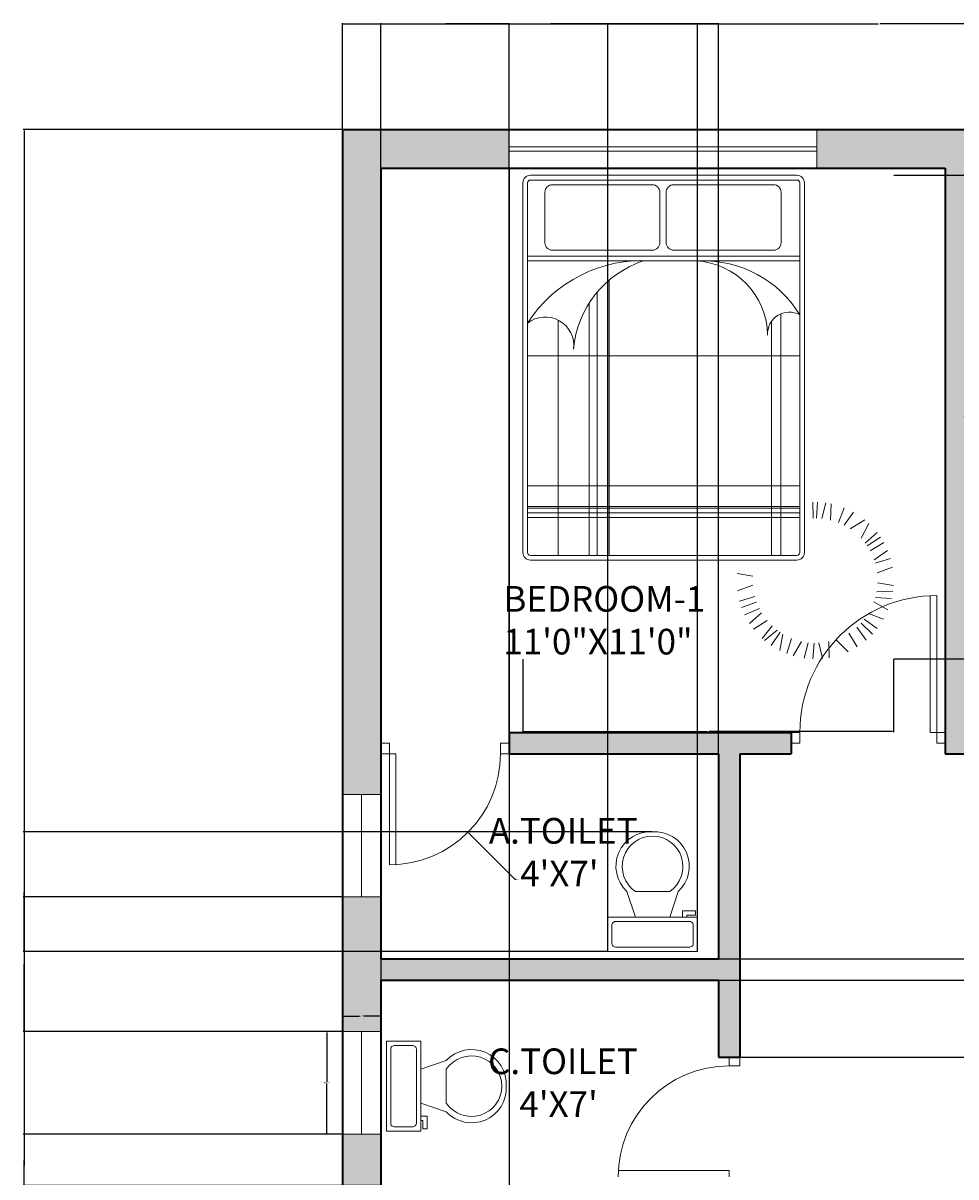
# Model space of a CAD drawing. Units: inches. Extents: x 126 to 477, y -70 to 465.
# Tile 3 of 5: x 126 to 344, y 195 to 465. Entities that reach past the tile are written whole.
import ezdxf

# ---------------------------------------------------------------- set-up
doc = ezdxf.new("R2010")
doc.units = ezdxf.units.IN
for name, color, linetype, lineweight in [('A-ANNO-DIMS', 2, 'Continuous', 18), ('A-AREA-IDEN', 7, 'Continuous', 20), ('A-DOOR', 4, 'Continuous', 20), ('A-FLOR-FIXT', 8, 'Continuous', 18), ('A-FURN', 8, 'Continuous', 18), ('A-GLAZ', 4, 'Continuous', 18), ('A-WALL', 7, 'Continuous', 35), ('A-WALL-PATT', 252, 'Continuous', 13)]:
    doc.layers.add(name, color=color, linetype=linetype, lineweight=lineweight)
doc.styles.get("Standard").update_dxf_attribs({"font": 'arial.ttf'})
doc.dimstyles.get("Standard").update_dxf_attribs({"dimtxt": 0.18, "dimasz": 0.18, "dimexe": 0.18, "dimexo": 0.0625, "dimgap": 0.09, "dimtad": 0, "dimtih": 1, "dimtoh": 1, "dimdec": 4, "dimzin": 0, "dimdsep": 46, "dimtxsty": 'Standard', "dimcen": 0.09, "dimadec": 0, "dimazin": 0, "dimtfac": 1, "dimtdec": 4, "dimtofl": 0, "dimtmove": 0, "dimatfit": 3, "dimfxl": 1, "dimtolj": 1, "dimtzin": 0, "dimarcsym": 0})

# ---------------------------------------------------------------- blocks, each defined once
blk = doc.blocks.new('*U6')
for p, q in [((9.5, -6), (9.5, -2)), ((-8, -8.5), (-8, -8)), ((-7, -8), (-7, -9.5)), ((-4, -8), (-6, -14)), ((4, -8), (6, -14)), ((-10, -8.5), (-8, -8.5)), ((-10, -9.5), (-10, -8.5)), ((-7, -9.5), (-10, -9.5)), ((4, -14), (-4, -14))]:
    blk.add_line(p, q)
blk.add_lwpolyline([(10.5, -8), (10.5, 0), (-10.5, 0), (-10.5, -8)], close=True)
for points in [[(-9.5, -2), (-9.5, -6)], [(8.5, -1), (-8.5, -1)], [(-8.5, -7), (8.5, -7)]]:
    blk.add_lwpolyline(points)
for centre, radius, start, end in [((-8.625, -1.875), 0.8839, 81.8699, 188.1301), ((8.625, -1.875), 0.8839, 351.8699, 98.1301), ((-8.625, -6.125), 0.8839, 171.869898, 278.1301), ((8.625, -6.125), 0.8839, 261.8699, 8.1301), ((-0.4772, -19.9188), 8.0953, 133.01722, 273.38), ((0.0374, -19.8731), 7.127, 124.50543, 269.7), ((-0.0373, -19.8731), 7.127, 270.3, 55.4946), ((0.4773, -19.9188), 8.0953, 266.62, 46.9828)]:
    blk.add_arc(centre, radius, start, end)
blk = doc.blocks.new('A$C20A07B91')
for p, q in [((0, 0.5668), (0, 2.5368)), ((0.025, 0.5668), (0.025, 2.5368)), ((0.04, 2.5768), (1.46, 2.5768)), ((0.04, 2.5518), (1.46, 2.5518)), ((0.1577, 2.5267), (0.6896, 2.5267)), ((0.8032, 2.5267), (1.3351, 2.5267)), ((1.475, 2.5368), (1.475, 0.5668)), ((1.5, 2.5368), (1.5, 0.5668)), ((0.1177, 2.2177), (0.1177, 2.4867)), ((0.7296, 2.4867), (0.7296, 2.2177)), ((0.7632, 2.2177), (0.7632, 2.4867)), ((1.3751, 2.4867), (1.3751, 2.2177)), ((0.6896, 2.1777), (0.1577, 2.1777)), ((1.3351, 2.1777), (0.8032, 2.1777)), ((1.475, 2.1455), (0.025, 2.1455)), ((1.475, 2.1208), (0.025, 2.1208)), ((0.4594, 2.0186), (0.4594, 0.5518)), ((0.3952, 1.9538), (0.3952, 0.5518)), ((0.3537, 1.8973), (0.3537, 0.5518)), ((0.1881, 1.8055), (0.1881, 0.5518)), ((1.325, 1.7998), (1.325, 0.5518)), ((1.3735, 1.8387), (1.3735, 0.5518)), ((1.475, 1.6146), (0.025, 1.6146)), ((1.475, 0.9216), (0.025, 0.9216)), ((1.475, 0.8127), (0.025, 0.8127)), ((1.475, 0.8028), (0.025, 0.8028)), ((1.5448, 0.8348), (1.5455, 0.7499)), ((1.5699, 0.8347), (1.5633, 0.7501)), ((1.6143, 0.831), (1.5932, 0.7481)), ((1.6427, 0.8261), (1.6378, 0.7402)), ((1.7121, 0.8051), (1.6806, 0.7263)), ((1.475, 0.778), (0.025, 0.778)), ((1.475, 0.7533), (0.025, 0.7533)), ((1.7614, 0.7816), (1.7107, 0.7125)), ((1.8218, 0.7404), (1.7431, 0.6933)), ((1.8424, 0.7223), (1.8011, 0.6437)), ((1.8863, 0.6743), (1.8232, 0.6171)), ((1.9045, 0.6491), (1.833, 0.6034)), ((1.9224, 0.6197), (1.8494, 0.5764)), ((1.9429, 0.5771), (1.8708, 0.5282)), ((1.46, 0.5518), (0.04, 0.5518)), ((1.46, 0.5268), (0.04, 0.5268)), ((1.9576, 0.5356), (1.8768, 0.5097)), ((1.1413, 0.4558), (1.2253, 0.4415)), ((1.9686, 0.4882), (1.8872, 0.4594)), ((1.1432, 0.3625), (1.2252, 0.3937)), ((1.9739, 0.3913), (1.8896, 0.4048)), ((1.1543, 0.3074), (1.2354, 0.3323)), ((1.9636, 0.322), (1.8777, 0.3283)), ((1.9708, 0.3609), (1.8845, 0.3578)), ((1.2446, 0.3031), (1.1649, 0.2741)), ((1.1813, 0.2354), (1.2596, 0.2685)), ((1.2719, 0.2461), (1.2078, 0.1886)), ((1.9448, 0.2622), (1.8701, 0.3046)), ((1.3016, 0.2043), (1.2293, 0.1587)), ((1.8616, 0.1317), (1.8013, 0.1913)), ((1.888, 0.1627), (1.8187, 0.2117)), ((1.8402, 0.2426), (1.9212, 0.2128)), ((1.328, 0.1761), (1.2751, 0.1095)), ((1.2875, 0.0985), (1.3538, 0.154)), ((1.37, 0.1423), (1.3226, 0.0719)), ((1.3681, 0.0451), (1.3852, 0.1325)), ((1.7812, 0.065), (1.736, 0.1369)), ((1.7796, 0.17), (1.8287, 0.1002)), ((1.4315, 0.1093), (1.4056, 0.0283)), ((1.44, 0.0166), (1.4837, 0.0929)), ((1.5197, 0.0868), (1.499, 0.0039)), ((1.5447, 0), (1.5511, 0.0847)), ((1.5756, 0.0852), (1.5955, 0.0016)), ((1.6305, 0.0929), (1.6312, 0.0064)), ((1.6678, 0.1036), (1.7332, 0.0388))]:
    blk.add_line(p, q)
for centre, radius, start, end in [((0.04, 2.5368), 0.04, 90, 180), ((0.04, 2.5368), 0.015, 90, 180), ((0.1577, 2.4867), 0.04, 90, 180), ((0.6896, 2.4867), 0.04, 0, 90), ((0.8032, 2.4867), 0.04, 90, 180), ((1.3351, 2.4867), 0.04, 0, 90), ((1.46, 2.5368), 0.04, 0, 90), ((1.46, 2.5368), 0.015, 0, 90), ((0.1577, 2.2177), 0.04, 180, 270), ((0.6896, 2.2177), 0.04, 270, 0), ((0.8032, 2.2177), 0.04, 180, 270), ((1.3351, 2.2177), 0.04, 270, 0), ((0.6351, 1.3977), 0.7248, 86.01998, 147.31517), ((0.8125, 1.604), 0.5445, 108.37185, 175.10395), ((0.9022, 1.72), 0.4013, 0.68408, 87.06887), ((0.9629, 1.5212), 0.5999, 31.38578, 91.94583), ((1.419, 1.7323), 0.1157, 61.08706, 183.75653), ((0.1193, 1.6701), 0.1519, 352.59612, 128.40132), ((0.04, 0.5668), 0.04, 180, 270), ((0.04, 0.5668), 0.015, 180, 270), ((1.46, 0.5668), 0.04, 270, 0), ((1.46, 0.5668), 0.015, 270, 0)]:
    blk.add_arc(centre, radius, start, end)
blk = doc.blocks.new('DOOR-SINGLE-36IN')
for p, q in [((2, 34.5), (2, 2.5)), ((3.5, 34.46), (3.5, 2.5)), ((2, 2.5), (0, 2.5)), ((0, 0), (2, 0)), ((2, 0), (2, 2.5)), ((2, 2.5), (3.5, 2.5)), ((34, 0), (34, 2.5)), ((34, 2.5), (36, 2.5)), ((36, 0), (34, 0))]:
    blk.add_line(p, q)
blk.add_arc((2, 2.5), 32, 0, 90)
blk = doc.blocks.new('WIN-72IN')
for p, q in [((0, 0), (0, 9)), ((72, 0), (72, 9)), ((72, 5), (0, 5)), ((72, 4), (0, 4))]:
    blk.add_line(p, q)
blk = doc.blocks.new('VENT-WIN-24IN')
for p, q in [((9, 24), (0, 24)), ((4.5, 24), (4.5, 0)), ((9, 0), (0, 0))]:
    blk.add_line(p, q)
blk = doc.blocks.new('*D15')
at = {"layer": 'A-ANNO-DIMS', "color": 0, "lineweight": -2, "transparency": 16777216}
for p, q in [((200.47, 228.88), (196.75, 228.88)), ((196.93, 228.7), (196.93, 217.06)), ((196.93, 205.06), (196.93, 216.7)), ((200.47, 204.88), (196.75, 204.88))]:
    blk.add_line(p, q, dxfattribs=at)
at = {"layer": 'A-ANNO-DIMS', "color": 0, "transparency": 16777216}
for points in [[(196.9, 228.7), (196.96, 228.7), (196.93, 228.88)], [(196.9, 205.06), (196.96, 205.06), (196.93, 204.88)]]:
    blk.add_solid(points, dxfattribs=at)
at = {"layer": 'Defpoints', "color": 0, "transparency": 16777216}
for p in [(196.93, 228.88), (200.53, 228.88), (200.53, 204.88)]:
    blk.add_point(p, dxfattribs=at)
at = {"layer": 'A-ANNO-DIMS', "color": 0, "transparency": 16777216, "insert": (196.93, 216.88), "char_height": 0.18, "attachment_point": 5}
blk.add_mtext('\\A1;VENT 24 TYP.', dxfattribs=at)
blk = doc.blocks.new('*D16')
at = {"layer": 'A-ANNO-DIMS', "color": 0, "lineweight": -2, "transparency": 16777216}
for p, q in [((200.53, 228.94), (200.53, 232.66)), ((200.71, 232.48), (204.58, 232.48)), ((209.35, 232.48), (205.49, 232.48)), ((209.53, 228.94), (209.53, 232.66))]:
    blk.add_line(p, q, dxfattribs=at)
at = {"layer": 'A-ANNO-DIMS', "color": 0, "transparency": 16777216}
for points in [[(200.71, 232.51), (200.71, 232.45), (200.53, 232.48)], [(209.35, 232.51), (209.35, 232.45), (209.53, 232.48)]]:
    blk.add_solid(points, dxfattribs=at)
at = {"layer": 'Defpoints', "color": 0, "transparency": 16777216}
for p in [(209.53, 232.48), (200.53, 228.88), (209.53, 228.88)]:
    blk.add_point(p, dxfattribs=at)
at = {"layer": 'A-ANNO-DIMS', "color": 0, "transparency": 16777216, "insert": (205.03, 232.48), "char_height": 0.18, "attachment_point": 5}
blk.add_mtext('\\A1;9 TYP.', dxfattribs=at)
blk = doc.blocks.new('*D19')
at = {"layer": 'A-ANNO-DIMS', "color": 0, "lineweight": -2, "transparency": 16777216}
for p, q in [((329.49, 429.2), (346.57, 429.2)), ((346.39, 429.02), (346.39, 372.81)), ((346.39, 316.23), (346.39, 372.44)), ((329.49, 316.05), (346.57, 316.05))]:
    blk.add_line(p, q, dxfattribs=at)
at = {"layer": 'A-ANNO-DIMS', "color": 0, "transparency": 16777216}
for points in [[(346.36, 429.02), (346.42, 429.02), (346.39, 429.2)], [(346.36, 316.23), (346.42, 316.23), (346.39, 316.05)]]:
    blk.add_solid(points, dxfattribs=at)
at = {"layer": 'Defpoints', "color": 0, "transparency": 16777216}
for p in [(329.42, 429.2), (346.39, 429.2), (329.42, 316.05)]:
    blk.add_point(p, dxfattribs=at)
at = {"layer": 'A-ANNO-DIMS', "color": 0, "transparency": 16777216, "insert": (346.39, 372.63), "char_height": 0.18, "attachment_point": 5}
blk.add_mtext('\\A1;BED GROUP 113', dxfattribs=at)
blk = doc.blocks.new('*D20')
at = {"layer": 'A-ANNO-DIMS', "color": 0, "lineweight": -2, "transparency": 16777216}
for p, q in [((242.75, 315.99), (242.75, 298.9)), ((329.42, 315.99), (329.42, 298.9)), ((242.93, 299.08), (285.87, 299.08)), ((329.24, 299.08), (286.31, 299.08))]:
    blk.add_line(p, q, dxfattribs=at)
at = {"layer": 'A-ANNO-DIMS', "color": 0, "transparency": 16777216}
for points in [[(242.93, 299.11), (242.93, 299.05), (242.75, 299.08)], [(329.24, 299.11), (329.24, 299.05), (329.42, 299.08)]]:
    blk.add_solid(points, dxfattribs=at)
at = {"layer": 'Defpoints', "color": 0, "transparency": 16777216}
for p in [(242.75, 316.05), (329.42, 316.05), (329.42, 299.08)]:
    blk.add_point(p, dxfattribs=at)
at = {"layer": 'A-ANNO-DIMS', "color": 0, "transparency": 16777216, "insert": (286.09, 299.08), "char_height": 0.18, "attachment_point": 5}
blk.add_mtext('\\A1;87', dxfattribs=at)
blk = doc.blocks.new('*D29')
at = {"layer": 'A-ANNO-DIMS', "color": 0, "lineweight": -2, "transparency": 16777216}
for p, q in [((200.53, 439.94), (200.53, 464.81)), ((200.71, 464.63), (325.76, 464.63)), ((451.35, 464.63), (326.31, 464.63)), ((451.53, 439.94), (451.53, 464.81))]:
    blk.add_line(p, q, dxfattribs=at)
at = {"layer": 'A-ANNO-DIMS', "color": 0, "transparency": 16777216}
for points in [[(200.71, 464.66), (200.71, 464.6), (200.53, 464.63)], [(451.35, 464.66), (451.35, 464.6), (451.53, 464.63)]]:
    blk.add_solid(points, dxfattribs=at)
at = {"layer": 'Defpoints', "color": 0, "transparency": 16777216}
for p in [(451.53, 464.63), (200.53, 439.88), (451.53, 439.88)]:
    blk.add_point(p, dxfattribs=at)
at = {"layer": 'A-ANNO-DIMS', "color": 0, "transparency": 16777216, "insert": (326.03, 464.63), "char_height": 0.18, "attachment_point": 5}
blk.add_mtext('\\A1;251', dxfattribs=at)
blk = doc.blocks.new('*D30')
at = {"layer": 'A-ANNO-DIMS', "color": 0, "lineweight": -2, "transparency": 16777216}
for p, q in [((200.47, 439.88), (125.92, 439.88)), ((126.1, 439.7), (126.1, 197.56)), ((126.1, -44.94), (126.1, 197.2)), ((200.47, -45.12), (125.92, -45.12))]:
    blk.add_line(p, q, dxfattribs=at)
at = {"layer": 'A-ANNO-DIMS', "color": 0, "transparency": 16777216}
for points in [[(126.07, 439.7), (126.13, 439.7), (126.1, 439.88)], [(126.07, -44.94), (126.13, -44.94), (126.1, -45.12)]]:
    blk.add_solid(points, dxfattribs=at)
at = {"layer": 'Defpoints', "color": 0, "transparency": 16777216}
for p in [(126.1, 439.88), (200.53, 439.88), (200.53, -45.12)]:
    blk.add_point(p, dxfattribs=at)
at = {"layer": 'A-ANNO-DIMS', "color": 0, "transparency": 16777216, "insert": (126.1, 197.38), "char_height": 0.18, "attachment_point": 5}
blk.add_mtext('\\A1;485', dxfattribs=at)
blk = doc.blocks.new('*D31')
at = {"layer": 'A-ANNO-DIMS', "color": 0, "lineweight": -2, "transparency": 16777216}
for p, q in [((209.53, 430.82), (209.53, -70.05)), ((239.53, 430.82), (239.53, -70.05)), ((209.71, -69.87), (224.31, -69.87)), ((239.35, -69.87), (224.75, -69.87))]:
    blk.add_line(p, q, dxfattribs=at)
at = {"layer": 'A-ANNO-DIMS', "color": 0, "transparency": 16777216}
for points in [[(209.71, -69.84), (209.71, -69.9), (209.53, -69.87)], [(239.35, -69.84), (239.35, -69.9), (239.53, -69.87)]]:
    blk.add_solid(points, dxfattribs=at)
at = {"layer": 'Defpoints', "color": 0, "transparency": 16777216}
for p in [(209.53, 430.88), (239.53, 430.88), (239.53, -69.87)]:
    blk.add_point(p, dxfattribs=at)
at = {"layer": 'A-ANNO-DIMS', "color": 0, "transparency": 16777216, "insert": (224.53, -69.87), "char_height": 0.18, "attachment_point": 5}
blk.add_mtext('\\A1;30', dxfattribs=at)
blk = doc.blocks.new('*D49')
at = {"layer": 'A-ANNO-DIMS', "color": 0, "lineweight": -2, "transparency": 16777216}
for p, q in [((209.53, 245.94), (209.53, 464.81)), ((209.71, 464.63), (248.81, 464.63)), ((288.35, 464.63), (249.25, 464.63)), ((288.53, 245.94), (288.53, 464.81))]:
    blk.add_line(p, q, dxfattribs=at)
at = {"layer": 'A-ANNO-DIMS', "color": 0, "transparency": 16777216}
for points in [[(209.71, 464.66), (209.71, 464.6), (209.53, 464.63)], [(288.35, 464.66), (288.35, 464.6), (288.53, 464.63)]]:
    blk.add_solid(points, dxfattribs=at)
at = {"layer": 'Defpoints', "color": 0, "transparency": 16777216}
for p in [(288.53, 464.63), (209.53, 245.88), (288.53, 245.88)]:
    blk.add_point(p, dxfattribs=at)
at = {"layer": 'A-ANNO-DIMS', "color": 0, "transparency": 16777216, "insert": (249.03, 464.63), "char_height": 0.18, "attachment_point": 5}
blk.add_mtext('\\A1;79', dxfattribs=at)
blk = doc.blocks.new('*D50')
at = {"layer": 'A-ANNO-DIMS', "color": 0, "lineweight": -2, "transparency": 16777216}
for p, q in [((209.53, 298.94), (209.53, 464.81)), ((209.71, 464.63), (224.31, 464.63)), ((239.35, 464.63), (224.75, 464.63)), ((239.53, 298.94), (239.53, 464.81))]:
    blk.add_line(p, q, dxfattribs=at)
at = {"layer": 'A-ANNO-DIMS', "color": 0, "transparency": 16777216}
for points in [[(209.71, 464.66), (209.71, 464.6), (209.53, 464.63)], [(239.35, 464.66), (239.35, 464.6), (239.53, 464.63)]]:
    blk.add_solid(points, dxfattribs=at)
at = {"layer": 'Defpoints', "color": 0, "transparency": 16777216}
for p in [(239.53, 464.63), (209.53, 298.88), (239.53, 298.88)]:
    blk.add_point(p, dxfattribs=at)
at = {"layer": 'A-ANNO-DIMS', "color": 0, "transparency": 16777216, "insert": (224.53, 464.63), "char_height": 0.18, "attachment_point": 5}
blk.add_mtext('\\A1;30', dxfattribs=at)
blk = doc.blocks.new('*D51')
at = {"layer": 'A-ANNO-DIMS', "color": 0, "lineweight": -2, "transparency": 16777216}
for p, q in [((293.6, 222.88), (476.46, 222.88)), ((476.28, 222.7), (476.28, 208.06)), ((476.28, 193.06), (476.28, 207.7)), ((293.6, 192.88), (476.46, 192.88))]:
    blk.add_line(p, q, dxfattribs=at)
at = {"layer": 'A-ANNO-DIMS', "color": 0, "transparency": 16777216}
for points in [[(476.25, 222.7), (476.31, 222.7), (476.28, 222.88)], [(476.25, 193.06), (476.31, 193.06), (476.28, 192.88)]]:
    blk.add_solid(points, dxfattribs=at)
at = {"layer": 'Defpoints', "color": 0, "transparency": 16777216}
for p in [(293.53, 222.88), (476.28, 222.88), (293.53, 192.88)]:
    blk.add_point(p, dxfattribs=at)
at = {"layer": 'A-ANNO-DIMS', "color": 0, "transparency": 16777216, "insert": (476.28, 207.88), "char_height": 0.18, "attachment_point": 5}
blk.add_mtext('\\A1;30', dxfattribs=at)
blk = doc.blocks.new('*D52')
at = {"layer": 'A-ANNO-DIMS', "color": 0, "lineweight": -2, "transparency": 16777216}
for p, q in [((200.47, 260.38), (125.92, 260.38)), ((126.1, 260.2), (126.1, 244.81)), ((126.1, 229.06), (126.1, 244.45)), ((200.47, 228.88), (125.92, 228.88))]:
    blk.add_line(p, q, dxfattribs=at)
at = {"layer": 'A-ANNO-DIMS', "color": 0, "transparency": 16777216}
for points in [[(126.07, 260.2), (126.13, 260.2), (126.1, 260.38)], [(126.07, 229.06), (126.13, 229.06), (126.1, 228.88)]]:
    blk.add_solid(points, dxfattribs=at)
at = {"layer": 'Defpoints', "color": 0, "transparency": 16777216}
for p in [(126.1, 260.38), (200.53, 260.38), (200.53, 228.88)]:
    blk.add_point(p, dxfattribs=at)
at = {"layer": 'A-ANNO-DIMS', "color": 0, "transparency": 16777216, "insert": (126.1, 244.63), "char_height": 0.18, "attachment_point": 5}
blk.add_mtext('\\A1;31.5', dxfattribs=at)
blk = doc.blocks.new('*D53')
at = {"layer": 'A-ANNO-DIMS', "color": 0, "lineweight": -2, "transparency": 16777216}
for p, q in [((200.47, 204.88), (125.92, 204.88)), ((126.1, 204.7), (126.1, 199.06)), ((126.1, 193.06), (126.1, 198.7)), ((209.47, 192.88), (125.92, 192.88))]:
    blk.add_line(p, q, dxfattribs=at)
at = {"layer": 'A-ANNO-DIMS', "color": 0, "transparency": 16777216}
for points in [[(126.07, 204.7), (126.13, 204.7), (126.1, 204.88)], [(126.07, 193.06), (126.13, 193.06), (126.1, 192.88)]]:
    blk.add_solid(points, dxfattribs=at)
at = {"layer": 'Defpoints', "color": 0, "transparency": 16777216}
for p in [(126.1, 204.88), (200.53, 204.88), (209.53, 192.88)]:
    blk.add_point(p, dxfattribs=at)
at = {"layer": 'A-ANNO-DIMS', "color": 0, "transparency": 16777216, "insert": (126.1, 198.88), "char_height": 0.18, "attachment_point": 5}
blk.add_mtext('\\A1;12', dxfattribs=at)
blk = doc.blocks.new('*D54')
at = {"layer": 'A-ANNO-DIMS', "color": 0, "lineweight": -2, "transparency": 16777216}
for p, q in [((288.6, 245.88), (476.46, 245.88)), ((476.28, 245.7), (476.28, 243.56)), ((476.28, 241.06), (476.28, 243.2)), ((288.6, 240.88), (476.46, 240.88))]:
    blk.add_line(p, q, dxfattribs=at)
at = {"layer": 'A-ANNO-DIMS', "color": 0, "transparency": 16777216}
for points in [[(476.25, 245.7), (476.31, 245.7), (476.28, 245.88)], [(476.25, 241.06), (476.31, 241.06), (476.28, 240.88)]]:
    blk.add_solid(points, dxfattribs=at)
at = {"layer": 'Defpoints', "color": 0, "transparency": 16777216}
for p in [(288.53, 245.88), (476.28, 245.88), (288.53, 240.88)]:
    blk.add_point(p, dxfattribs=at)
at = {"layer": 'A-ANNO-DIMS', "color": 0, "transparency": 16777216, "insert": (476.28, 243.38), "char_height": 0.18, "attachment_point": 5}
blk.add_mtext('\\A1;5', dxfattribs=at)
blk = doc.blocks.new('*D55')
at = {"layer": 'A-ANNO-DIMS', "color": 0, "lineweight": -2, "transparency": 16777216}
for p, q in [((262.59, 247.7), (262.59, 464.81)), ((262.77, 464.63), (272.89, 464.63)), ((283.41, 464.63), (273.29, 464.63)), ((283.59, 247.7), (283.59, 464.81))]:
    blk.add_line(p, q, dxfattribs=at)
at = {"layer": 'A-ANNO-DIMS', "color": 0, "transparency": 16777216}
for points in [[(262.77, 464.66), (262.77, 464.6), (262.59, 464.63)], [(283.41, 464.66), (283.41, 464.6), (283.59, 464.63)]]:
    blk.add_solid(points, dxfattribs=at)
at = {"layer": 'Defpoints', "color": 0, "transparency": 16777216}
for p in [(283.59, 464.63), (262.59, 247.63), (283.59, 247.63)]:
    blk.add_point(p, dxfattribs=at)
at = {"layer": 'A-ANNO-DIMS', "color": 0, "transparency": 16777216, "insert": (273.09, 464.63), "char_height": 0.18, "attachment_point": 5}
blk.add_mtext('\\A1;21', dxfattribs=at)
blk = doc.blocks.new('*D56')
at = {"layer": 'A-ANNO-DIMS', "color": 0, "lineweight": -2, "transparency": 16777216}
for p, q in [((273.03, 275.63), (125.92, 275.63)), ((126.1, 275.45), (126.1, 261.82)), ((126.1, 247.81), (126.1, 261.45)), ((262.53, 247.63), (125.92, 247.63))]:
    blk.add_line(p, q, dxfattribs=at)
at = {"layer": 'A-ANNO-DIMS', "color": 0, "transparency": 16777216}
for points in [[(126.07, 275.45), (126.13, 275.45), (126.1, 275.63)], [(126.07, 247.81), (126.13, 247.81), (126.1, 247.63)]]:
    blk.add_solid(points, dxfattribs=at)
at = {"layer": 'Defpoints', "color": 0, "transparency": 16777216}
for p in [(126.1, 275.63), (273.09, 275.63), (262.59, 247.63)]:
    blk.add_point(p, dxfattribs=at)
at = {"layer": 'A-ANNO-DIMS', "color": 0, "transparency": 16777216, "insert": (126.1, 261.63), "char_height": 0.18, "attachment_point": 5}
blk.add_mtext('\\A1;28', dxfattribs=at)
blk = doc.blocks.new('*D57')
at = {"layer": 'A-ANNO-DIMS', "color": 0, "lineweight": -2, "transparency": 16777216}
for p, q in [((211.44, 293.88), (211.62, 293.88)), ((211.53, 293.79), (211.53, 293.97)), ((240.95, 264.47), (230.05, 275.37)), ((241.13, 264.47), (240.95, 264.47))]:
    blk.add_line(p, q, dxfattribs=at)
at = {"layer": 'A-ANNO-DIMS', "color": 0, "transparency": 16777216}
blk.add_solid([(230.07, 275.39), (230.02, 275.35), (229.92, 275.5)], dxfattribs=at)
at = {"layer": 'Defpoints', "color": 0, "transparency": 16777216}
for p in [(211.53, 293.88), (229.92, 275.5)]:
    blk.add_point(p, dxfattribs=at)
at = {"layer": 'A-ANNO-DIMS', "color": 0, "transparency": 16777216, "insert": (241.63, 264.47), "char_height": 0.18, "attachment_point": 5}
blk.add_mtext('\\A1;2X R26', dxfattribs=at)

msp = doc.modelspace()

# ---------------------------------------------------------------- hatches: boundary and pattern name
at = {"layer": 'A-WALL-PATT'}
h = msp.add_hatch(color=256, dxfattribs=at)
h.dxf.hatch_style = 1
h.paths.add_polyline_path([(239.5333, 439.8806), (200.5333, 439.8806), (200.5333, 284.3806), (209.5333, 284.3806), (209.5333, 298.8806), (209.5333, 430.8806), (239.5333, 430.8806)])
h = msp.add_hatch(color=256, dxfattribs=at)
h.dxf.hatch_style = 1
h.paths.add_polyline_path([(346.5333, 430.8806), (358.5333, 430.8806), (358.5333, 439.8806), (311.5333, 439.8806), (311.5333, 430.8806), (341.5333, 430.8806), (341.5333, 293.8806), (346.5333, 293.8806)])
h = msp.add_hatch(color=256, dxfattribs=at)
h.dxf.hatch_style = 1
h.paths.add_polyline_path([(293.5333, 293.8806), (305.5333, 293.8806), (305.5333, 298.8806), (239.5333, 298.8806), (239.5333, 293.8806), (288.5333, 293.8806), (288.5333, 245.8806), (209.5333, 245.8806), (209.5333, 260.3806), (200.5333, 260.3806), (200.5333, 228.8806), (209.5333, 228.8806), (209.5333, 240.8806), (288.5333, 240.8806), (288.5333, 222.8806), (293.5333, 222.8806)])
h = msp.add_hatch(color=256, dxfattribs=at)
h.dxf.hatch_style = 1
h.paths.add_polyline_path([(334.5333, -4.1194), (329.5333, -4.1194), (329.5333, -40.1194), (317.5333, -40.1194), (317.5333, -45.1194), (334.5333, -45.1194)])
h.paths.add_polyline_path([(205.5333, 58.8806), (233.5333, 58.8806), (233.5333, 67.8806), (209.5333, 67.8806), (209.5333, 187.8806), (293.5333, 187.8806), (293.5333, 192.8806), (209.5333, 192.8806), (209.5333, 204.8806), (200.5333, 204.8806), (200.5333, -45.1194), (209.5333, -45.1194), (209.5333, -40.1194), (205.5333, -40.1194)])

# ---------------------------------------------------------------- linework, layer by layer
at = {"layer": 'A-DOOR'}
for p, q in [((209.5333, 296.3806), (211.5333, 296.3806)), ((211.5333, 296.3806), (211.5333, 293.8806)), ((239.5333, 296.3806), (237.5333, 296.3806)), ((237.5333, 296.3806), (237.5333, 293.8806)), ((211.5333, 293.8806), (209.5333, 293.8806)), ((211.5333, 267.8806), (211.5333, 293.8806)), ((211.5333, 293.8806), (213.0333, 293.8806)), ((213.0333, 267.8806), (213.0333, 293.8806)), ((237.5333, 293.8806), (239.5333, 293.8806)), ((291.0333, 222.8806), (291.0333, 220.8806)), ((293.5333, 220.8806), (293.5333, 222.8806)), ((291.0333, 220.8806), (293.5333, 220.8806)), ((265.0766, 196.3806), (291.0333, 196.3806)), ((291.0333, 194.8806), (291.0333, 196.3806))]:
    msp.add_line(p, q, dxfattribs=at)
for centre, start, end in [((211.5333, 293.8806), 270, 0), ((291.0333, 194.8806), 90, 180)]:
    msp.add_arc(centre, 26, start, end, dxfattribs=at)
at = {"layer": 'A-WALL'}
for p, q in [((200.5333, 439.8806), (200.5333, -45.1194)), ((200.5333, 439.8806), (451.5333, 439.8806)), ((209.5333, 430.8806), (209.5333, 298.8806)), ((209.5333, 430.8806), (341.5333, 430.8806)), ((209.5333, 430.8806), (209.5333, 298.8806)), ((341.5333, 430.8806), (341.5333, 293.8806)), ((209.5333, 298.8806), (209.5333, 245.8806)), ((239.5333, 298.8806), (305.5333, 298.8806)), ((239.5333, 298.8806), (239.5333, 293.8806)), ((305.5333, 298.8806), (305.5333, 293.8806)), ((239.5333, 293.8806), (288.5333, 293.8806)), ((288.5333, 293.8806), (288.5333, 245.8806)), ((293.5333, 293.8806), (293.5333, 222.8806)), ((293.5333, 293.8806), (305.5333, 293.8806)), ((341.5333, 293.8806), (346.5333, 293.8806)), ((209.5333, 245.8806), (288.5333, 245.8806)), ((209.5333, 240.8806), (288.5333, 240.8806)), ((209.5333, 240.8806), (209.5333, 192.8806)), ((288.5333, 240.8806), (288.5333, 222.8806)), ((288.5333, 222.8806), (293.5333, 222.8806))]:
    msp.add_line(p, q, dxfattribs=at)

# ---------------------------------------------------------------- block references
at = {"layer": 'A-DOOR', "extrusion": (0, 0, -1), "zscale": -1}
msp.add_blockref('DOOR-SINGLE-36IN', (-341.5333, 296.3806), dxfattribs=at)
at = {"layer": 'A-FLOR-FIXT'}
for p, rotation in [((273.0888, 247.6348), 180), ((210.8501, 216.1135), 90)]:
    msp.add_blockref('*U6', p, dxfattribs=dict(at, rotation=rotation))
at = {"layer": 'A-FURN', "xscale": 43.90860666867045, "yscale": 43.90860666867045, "zscale": 43.90860666867045}
msp.add_blockref('A$C20A07B91', (242.753, 316.0525), dxfattribs=at)
at = {"layer": 'A-GLAZ'}
for name, p in [('WIN-72IN', (239.5333, 430.8806)), ('VENT-WIN-24IN', (200.5333, 260.3806)), ('VENT-WIN-24IN', (200.5333, 204.8806))]:
    msp.add_blockref(name, p, dxfattribs=at)

# ---------------------------------------------------------------- texts
at = {"layer": 'A-AREA-IDEN', "char_height": 6, "attachment_point": 1}
for s, width, insert in [('BEDROOM-1\\P11\'0"X11\'0"', 74.074101, (238.1898, 333.1078)), ("A.TOILET\\P    4'X7'", 64.633583, (234.7924, 278.8373)), ("C.TOILET\\P    4'X7'", 64.633583, (234.6109, 224.9331))]:
    msp.add_mtext_dynamic_manual_height_columns(s, width=width, gutter_width=12.5, heights=[0], dxfattribs=dict(at, insert=insert))

# ---------------------------------------------------------------- dimensions: what is measured, and where the dimension line sits
at = {"layer": 'A-ANNO-DIMS'}
for base, p1, p2, picture, middle in [((451.5333, 464.6306), (200.5333, 439.8806), (451.5333, 439.8806), '*D29', (326.0333, 464.6306)), ((288.5333, 464.6306), (209.5333, 245.8806), (288.5333, 245.8806), '*D49', (249.0333, 464.6306)), ((239.5333, 464.6306), (209.5333, 298.8806), (239.5333, 298.8806), '*D50', (224.5333, 464.6306)), ((283.5888, 464.6306), (262.5888, 247.6348), (283.5888, 247.6348), '*D55', (273.0888, 464.6306)), ((239.5333, -69.8694), (209.5333, 430.8806), (239.5333, 430.8806), '*D31', (224.5333, -69.8694)), ((329.4226, 299.0808), (242.753, 316.0525), (329.4226, 316.0525), '*D20', (286.0878, 299.0808))]:
    dim = msp.add_linear_dim(base=base, p1=p1, p2=p2, dimstyle='Standard', override={"dimdec": 0, "dimlfac": 1, "dimrnd": 0, "dimzin": 0, "dimdsep": 46, "dimlunit": 2}, dxfattribs=at)
    dim.commit()
    dim.dimension.update_dxf_attribs({"geometry": picture, "text_midpoint": middle})
for base, p1, p2, override, picture, middle in [((126.1001, 439.8806), (200.5333, -45.1194), (200.5333, 439.8806), {"dimdec": 0, "dimlfac": 1, "dimrnd": 0, "dimzin": 0, "dimdsep": 46, "dimlunit": 2}, '*D30', (126.1001, 197.3806)), ((126.1001, 275.6348), (262.5888, 247.6348), (273.0887, 275.6348), {"dimdec": 0, "dimlfac": 1, "dimrnd": 0, "dimzin": 0, "dimdsep": 46, "dimlunit": 2}, '*D56', (126.1001, 261.6348)), ((126.1001, 260.3806), (200.5333, 228.8806), (200.5333, 260.3806), {"dimdec": 1, "dimlfac": 1, "dimrnd": 0, "dimzin": 0, "dimdsep": 46, "dimlunit": 2}, '*D52', (126.1001, 244.6306)), ((476.2833, 245.8806), (288.5333, 240.8806), (288.5333, 245.8806), {"dimdec": 0, "dimlfac": 1, "dimrnd": 0, "dimzin": 0, "dimdsep": 46, "dimlunit": 2}, '*D54', (476.2833, 243.3806)), ((476.2833, 222.8806), (293.5333, 192.8806), (293.5333, 222.8806), {"dimdec": 0, "dimlfac": 1, "dimrnd": 0, "dimzin": 0, "dimdsep": 46, "dimlunit": 2}, '*D51', (476.2833, 207.8806)), ((126.1001, 204.8806), (209.5333, 192.8806), (200.5333, 204.8806), {"dimdec": 0, "dimlfac": 1, "dimrnd": 0, "dimzin": 0, "dimdsep": 46, "dimlunit": 2}, '*D53', (126.1001, 198.8806))]:
    dim = msp.add_linear_dim(base=base, p1=p1, p2=p2, angle=90, dimstyle='Standard', override=override, dxfattribs=at)
    dim.commit()
    dim.dimension.update_dxf_attribs({"geometry": picture, "text_midpoint": middle})
for base, p1, p2, text, picture, middle in [((346.3943, 429.1976), (329.4226, 316.0525), (329.4226, 429.1976), 'BED GROUP <>', '*D19', (346.3943, 372.6251)), ((196.9333, 228.8806), (200.5333, 204.8806), (200.5333, 228.8806), 'VENT <> TYP.', '*D15', (196.9333, 216.8806))]:
    dim = msp.add_linear_dim(base=base, p1=p1, p2=p2, angle=90, text=text, dimstyle='Standard', override={"dimdec": 0, "dimlfac": 1, "dimrnd": 0, "dimzin": 0, "dimdsep": 46, "dimlunit": 2}, dxfattribs=at)
    dim.commit()
    dim.dimension.update_dxf_attribs({"geometry": picture, "text_midpoint": middle})
dim = msp.add_radius_dim(center=(211.5333, 293.8806), mpoint=(229.9181, 275.4959), text='2X <>', dimstyle='Standard', override={"dimdec": 0, "dimlfac": 1, "dimrnd": 0, "dimzin": 0, "dimdsep": 46, "dimlunit": 2}, dxfattribs=at)
dim.commit()
dim.dimension.update_dxf_attribs({"geometry": '*D57', "text_midpoint": (241.6289, 264.465), "dimtype": 164})
dim = msp.add_linear_dim(base=(209.5333, 232.4806), p1=(200.5333, 228.8806), p2=(209.5333, 228.8806), text='<> TYP.', dimstyle='Standard', override={"dimdec": 0, "dimlfac": 1, "dimrnd": 0, "dimzin": 0, "dimdsep": 46, "dimlunit": 2}, dxfattribs=at)
dim.commit()
dim.dimension.update_dxf_attribs({"geometry": '*D16', "text_midpoint": (205.0333, 232.4806)})

doc.saveas('drawing.dxf')
